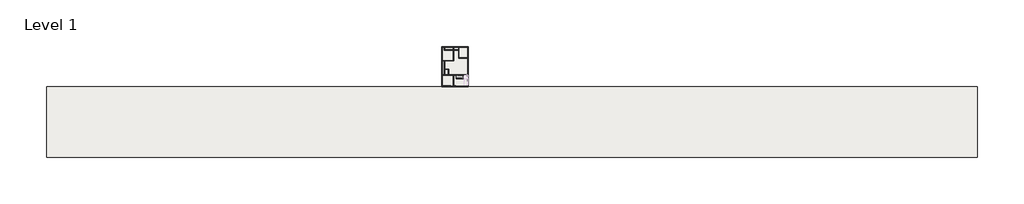
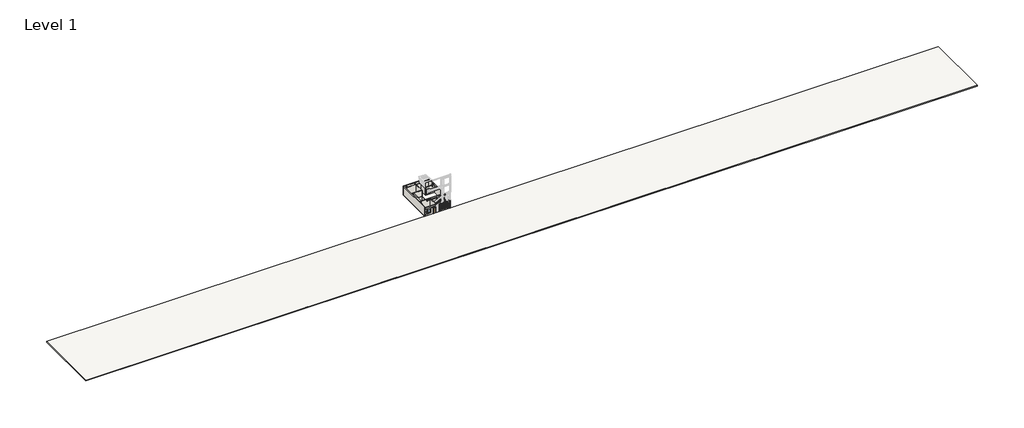
# One storey, part 1 of 2: 19 walls, 2 slabs, 1 door, 1 railing, 1 window.
"""IFC4 building model written with IfcOpenShell, lengths in millimetres."""

from ifc_helpers import new_model, si_unit, frame, origin, origin_with_axes, place, context, project, spatial, polyline, outline, extrude, faceted_brep, transform, mapped, element, save
from components import door_5e1232af, fixed_4x3_c1f32544

model = new_model("IFC4")

# Units and contexts
model_context = context("Model", 3, world=origin())
ifc_project = project(units=[si_unit("LENGTHUNIT", "METRE", prefix="MILLI")], contexts=[model_context])

# Site, building, storey
site = spatial("IfcSite", under=ifc_project)
building = spatial("IfcBuilding", under=site)
storey = spatial("IfcBuildingStorey", under=building, Name="Level 1", Elevation=0.0)

# Door
placement = place(None, origin())
door_shape = door_5e1232af(model_context)
element("IfcDoor", 1, ObjectType="Single-Flush : 30\" x 84\"", at=placement, inside=storey, context=model_context, shape_type="MappedRepresentation", body=[
    mapped(door_shape, transform((-2008.66646, -4503.4834702, 0.0), x_axis=(1.0, 0.0, 0.0), y_axis=(0.0, 1.0, 0.0), z_axis=(0.0, 0.0, 1.0))),
])

# Railing
element("IfcRailing", 2, ObjectType="Handrail - Rectangular", at=placement, inside=storey, context=model_context, shape_type="SolidModel", body=[
    faceted_brep([(-459.26646, -1798.3834702, 1066.8), (-459.26646, -1798.3834702, 1008.9343477), (-459.26646, -1849.1834702, 1008.9343477), (-459.26646, -1849.1834702, 1066.8), (2334.73354, -1798.3834702, 2590.8), (2347.687236, -1798.3834702, 2540.0), (2347.687236, -1849.1834702, 2540.0), (2334.73354, -1849.1834702, 2590.8), (2436.33354, -1798.3834702, 2590.8), (2436.33354, -1849.1834702, 2590.8), (2436.33354, -1849.1834702, 2540.0), (2436.33354, -1798.3834702, 2540.0)], [[[0, 1, 2, 3]], [[1, 0, 4, 5]], [[2, 1, 5, 6]], [[3, 2, 6, 7]], [[0, 3, 7, 4]], [[8, 9, 10, 11]], [[5, 4, 8, 11]], [[6, 5, 11, 10]], [[7, 6, 10, 9]], [[4, 7, 9, 8]]]),
    faceted_brep([(2436.33354, -1849.1834702, 2641.6), (2436.33354, -1849.1834702, 2528.0077467), (2385.53354, -1849.1834702, 2528.0077467), (2385.53354, -1849.1834702, 2641.6), (2436.33354, -1899.9834702, 2743.2), (2436.33354, -1938.2955084, 2706.231823), (2385.53354, -1938.2955084, 2706.231823), (2385.53354, -1899.9834702, 2743.2), (2436.33354, -4135.1834702, 3962.4), (2385.53354, -4135.1834702, 3962.4), (2385.53354, -4135.1834702, 3904.5343477), (2436.33354, -4135.1834702, 3904.5343477)], [[[0, 1, 2, 3]], [[1, 0, 4, 5]], [[2, 1, 5, 6]], [[3, 2, 6, 7]], [[0, 3, 7, 4]], [[8, 9, 10, 11]], [[5, 4, 8, 11]], [[6, 5, 11, 10]], [[7, 6, 10, 9]], [[4, 7, 9, 8]]]),
    extrude(outline(polyline([(-4043.1084702, 3854.3116204), (-4024.0584702, 3843.9207113), (-4024.0584702, 2895.6), (-4043.1084702, 2895.6), (-4043.1084702, 3854.3116204)])), frame((2401.40854, 0.0, 0.0), z_axis=(1.0, 0.0, 0.0), x_axis=(0.0, 1.0, 0.0)), (0.0, 0.0, 1.0), 19.05),
    extrude(outline(polyline([(-3941.5084702, 3798.8934386), (-3922.4584702, 3788.5025295), (-3922.4584702, 2895.6), (-3941.5084702, 2895.6), (-3941.5084702, 3798.8934386)])), frame((2401.40854, 0.0, 0.0), z_axis=(1.0, 0.0, 0.0), x_axis=(0.0, 1.0, 0.0)), (0.0, 0.0, 1.0), 19.05),
    extrude(outline(polyline([(-3839.9084702, 3743.4752568), (-3820.8584702, 3733.0843477), (-3820.8584702, 2743.2), (-3839.9084702, 2743.2), (-3839.9084702, 3743.4752568)])), frame((2401.40854, 0.0, 0.0), z_axis=(1.0, 0.0, 0.0), x_axis=(0.0, 1.0, 0.0)), (0.0, 0.0, 1.0), 19.05),
    extrude(outline(polyline([(-3738.3084702, 3688.0570749), (-3719.2584702, 3677.6661659), (-3719.2584702, 2743.2), (-3738.3084702, 2743.2), (-3738.3084702, 3688.0570749)])), frame((2401.40854, 0.0, 0.0), z_axis=(1.0, 0.0, 0.0), x_axis=(0.0, 1.0, 0.0)), (0.0, 0.0, 1.0), 19.05),
    extrude(outline(polyline([(-3636.7084702, 3632.6388931), (-3617.6584702, 3622.247984), (-3617.6584702, 2743.2), (-3636.7084702, 2743.2), (-3636.7084702, 3632.6388931)])), frame((2401.40854, 0.0, 0.0), z_axis=(1.0, 0.0, 0.0), x_axis=(0.0, 1.0, 0.0)), (0.0, 0.0, 1.0), 19.05),
    extrude(outline(polyline([(-3535.1084702, 3577.2207113), (-3516.0584702, 3566.8298022), (-3516.0584702, 2590.8), (-3535.1084702, 2590.8), (-3535.1084702, 3577.2207113)])), frame((2401.40854, 0.0, 0.0), z_axis=(1.0, 0.0, 0.0), x_axis=(0.0, 1.0, 0.0)), (0.0, 0.0, 1.0), 19.05),
    extrude(outline(polyline([(-3433.5084702, 3521.8025295), (-3414.4584702, 3511.4116204), (-3414.4584702, 2590.8), (-3433.5084702, 2590.8), (-3433.5084702, 3521.8025295)])), frame((2401.40854, 0.0, 0.0), z_axis=(1.0, 0.0, 0.0), x_axis=(0.0, 1.0, 0.0)), (0.0, 0.0, 1.0), 19.05),
    extrude(outline(polyline([(-3331.9084702, 3466.3843477), (-3312.8584702, 3455.9934386), (-3312.8584702, 2590.8), (-3331.9084702, 2590.8), (-3331.9084702, 3466.3843477)])), frame((2401.40854, 0.0, 0.0), z_axis=(1.0, 0.0, 0.0), x_axis=(0.0, 1.0, 0.0)), (0.0, 0.0, 1.0), 19.05),
    extrude(outline(polyline([(-3230.3084702, 3410.9661659), (-3211.2584702, 3400.5752568), (-3211.2584702, 2438.4), (-3230.3084702, 2438.4), (-3230.3084702, 3410.9661659)])), frame((2401.40854, 0.0, 0.0), z_axis=(1.0, 0.0, 0.0), x_axis=(0.0, 1.0, 0.0)), (0.0, 0.0, 1.0), 19.05),
    extrude(outline(polyline([(-3128.7084702, 3355.547984), (-3109.6584702, 3345.1570749), (-3109.6584702, 2438.4), (-3128.7084702, 2438.4), (-3128.7084702, 3355.547984)])), frame((2401.40854, 0.0, 0.0), z_axis=(1.0, 0.0, 0.0), x_axis=(0.0, 1.0, 0.0)), (0.0, 0.0, 1.0), 19.05),
    extrude(outline(polyline([(-3027.1084702, 3300.1298022), (-3008.0584702, 3289.7388931), (-3008.0584702, 2438.4), (-3027.1084702, 2438.4), (-3027.1084702, 3300.1298022)])), frame((2401.40854, 0.0, 0.0), z_axis=(1.0, 0.0, 0.0), x_axis=(0.0, 1.0, 0.0)), (0.0, 0.0, 1.0), 19.05),
    extrude(outline(polyline([(-2925.5084702, 3244.7116204), (-2906.4584702, 3234.3207113), (-2906.4584702, 2286.0), (-2925.5084702, 2286.0), (-2925.5084702, 3244.7116204)])), frame((2401.40854, 0.0, 0.0), z_axis=(1.0, 0.0, 0.0), x_axis=(0.0, 1.0, 0.0)), (0.0, 0.0, 1.0), 19.05),
    extrude(outline(polyline([(-2823.9084702, 3189.2934386), (-2804.8584702, 3178.9025295), (-2804.8584702, 2286.0), (-2823.9084702, 2286.0), (-2823.9084702, 3189.2934386)])), frame((2401.40854, 0.0, 0.0), z_axis=(1.0, 0.0, 0.0), x_axis=(0.0, 1.0, 0.0)), (0.0, 0.0, 1.0), 19.05),
    extrude(outline(polyline([(-2722.3084702, 3133.8752568), (-2703.2584702, 3123.4843477), (-2703.2584702, 2133.6), (-2722.3084702, 2133.6), (-2722.3084702, 3133.8752568)])), frame((2401.40854, 0.0, 0.0), z_axis=(1.0, 0.0, 0.0), x_axis=(0.0, 1.0, 0.0)), (0.0, 0.0, 1.0), 19.05),
    extrude(outline(polyline([(-2620.7084702, 3078.4570749), (-2601.6584702, 3068.0661659), (-2601.6584702, 2133.6), (-2620.7084702, 2133.6), (-2620.7084702, 3078.4570749)])), frame((2401.40854, 0.0, 0.0), z_axis=(1.0, 0.0, 0.0), x_axis=(0.0, 1.0, 0.0)), (0.0, 0.0, 1.0), 19.05),
    extrude(outline(polyline([(-2519.1084702, 3023.0388931), (-2500.0584702, 3012.647984), (-2500.0584702, 2133.6), (-2519.1084702, 2133.6), (-2519.1084702, 3023.0388931)])), frame((2401.40854, 0.0, 0.0), z_axis=(1.0, 0.0, 0.0), x_axis=(0.0, 1.0, 0.0)), (0.0, 0.0, 1.0), 19.05),
    extrude(outline(polyline([(-2417.5084702, 2967.6207113), (-2398.4584702, 2957.2298022), (-2398.4584702, 1981.2), (-2417.5084702, 1981.2), (-2417.5084702, 2967.6207113)])), frame((2401.40854, 0.0, 0.0), z_axis=(1.0, 0.0, 0.0), x_axis=(0.0, 1.0, 0.0)), (0.0, 0.0, 1.0), 19.05),
    extrude(outline(polyline([(-2315.9084702, 2912.2025295), (-2296.8584702, 2901.8116204), (-2296.8584702, 1981.2), (-2315.9084702, 1981.2), (-2315.9084702, 2912.2025295)])), frame((2401.40854, 0.0, 0.0), z_axis=(1.0, 0.0, 0.0), x_axis=(0.0, 1.0, 0.0)), (0.0, 0.0, 1.0), 19.05),
    extrude(outline(polyline([(-2214.3084702, 2856.7843477), (-2195.2584702, 2846.3934386), (-2195.2584702, 1981.2), (-2214.3084702, 1981.2), (-2214.3084702, 2856.7843477)])), frame((2401.40854, 0.0, 0.0), z_axis=(1.0, 0.0, 0.0), x_axis=(0.0, 1.0, 0.0)), (0.0, 0.0, 1.0), 19.05),
    extrude(outline(polyline([(-2112.7084702, 2801.3661659), (-2093.6584702, 2790.9752568), (-2093.6584702, 1828.8), (-2112.7084702, 1828.8), (-2112.7084702, 2801.3661659)])), frame((2401.40854, 0.0, 0.0), z_axis=(1.0, 0.0, 0.0), x_axis=(0.0, 1.0, 0.0)), (0.0, 0.0, 1.0), 19.05),
    extrude(outline(polyline([(-2011.1084702, 2745.947984), (-1992.0584702, 2735.5570749), (-1992.0584702, 1828.8), (-2011.1084702, 1828.8), (-2011.1084702, 2745.947984)])), frame((2401.40854, 0.0, 0.0), z_axis=(1.0, 0.0, 0.0), x_axis=(0.0, 1.0, 0.0)), (0.0, 0.0, 1.0), 19.05),
    extrude(outline(polyline([(2510.4207113, 2293.45854), (2500.0298022, 2274.40854), (1524.0, 2274.40854), (1524.0, 2293.45854), (2510.4207113, 2293.45854)])), frame((0.0, -1833.3084702, 0.0), z_axis=(0.0, 1.0, 0.0), x_axis=(0.0, 0.0, 1.0)), (0.0, 0.0, 1.0), 19.05),
    extrude(outline(polyline([(2455.0025295, 2191.85854), (2444.6116204, 2172.80854), (1524.0, 2172.80854), (1524.0, 2191.85854), (2455.0025295, 2191.85854)])), frame((0.0, -1833.3084702, 0.0), z_axis=(0.0, 1.0, 0.0), x_axis=(0.0, 0.0, 1.0)), (0.0, 0.0, 1.0), 19.05),
    extrude(outline(polyline([(2399.5843477, 2090.25854), (2389.1934386, 2071.20854), (1524.0, 2071.20854), (1524.0, 2090.25854), (2399.5843477, 2090.25854)])), frame((0.0, -1833.3084702, 0.0), z_axis=(0.0, 1.0, 0.0), x_axis=(0.0, 0.0, 1.0)), (0.0, 0.0, 1.0), 19.05),
    extrude(outline(polyline([(2344.1661659, 1988.65854), (2333.7752568, 1969.60854), (1371.6, 1969.60854), (1371.6, 1988.65854), (2344.1661659, 1988.65854)])), frame((0.0, -1833.3084702, 0.0), z_axis=(0.0, 1.0, 0.0), x_axis=(0.0, 0.0, 1.0)), (0.0, 0.0, 1.0), 19.05),
    extrude(outline(polyline([(2288.747984, 1887.05854), (2278.3570749, 1868.00854), (1371.6, 1868.00854), (1371.6, 1887.05854), (2288.747984, 1887.05854)])), frame((0.0, -1833.3084702, 0.0), z_axis=(0.0, 1.0, 0.0), x_axis=(0.0, 0.0, 1.0)), (0.0, 0.0, 1.0), 19.05),
    extrude(outline(polyline([(2233.3298022, 1785.45854), (2222.9388931, 1766.40854), (1371.6, 1766.40854), (1371.6, 1785.45854), (2233.3298022, 1785.45854)])), frame((0.0, -1833.3084702, 0.0), z_axis=(0.0, 1.0, 0.0), x_axis=(0.0, 0.0, 1.0)), (0.0, 0.0, 1.0), 19.05),
    extrude(outline(polyline([(2177.9116204, 1683.85854), (2167.5207113, 1664.80854), (1219.2, 1664.80854), (1219.2, 1683.85854), (2177.9116204, 1683.85854)])), frame((0.0, -1833.3084702, 0.0), z_axis=(0.0, 1.0, 0.0), x_axis=(0.0, 0.0, 1.0)), (0.0, 0.0, 1.0), 19.05),
    extrude(outline(polyline([(2122.4934386, 1582.25854), (2112.1025295, 1563.20854), (1219.2, 1563.20854), (1219.2, 1582.25854), (2122.4934386, 1582.25854)])), frame((0.0, -1833.3084702, 0.0), z_axis=(0.0, 1.0, 0.0), x_axis=(0.0, 0.0, 1.0)), (0.0, 0.0, 1.0), 19.05),
    extrude(outline(polyline([(2067.0752568, 1480.65854), (2056.6843477, 1461.60854), (1066.8, 1461.60854), (1066.8, 1480.65854), (2067.0752568, 1480.65854)])), frame((0.0, -1833.3084702, 0.0), z_axis=(0.0, 1.0, 0.0), x_axis=(0.0, 0.0, 1.0)), (0.0, 0.0, 1.0), 19.05),
    extrude(outline(polyline([(2011.6570749, 1379.05854), (2001.2661659, 1360.00854), (1066.8, 1360.00854), (1066.8, 1379.05854), (2011.6570749, 1379.05854)])), frame((0.0, -1833.3084702, 0.0), z_axis=(0.0, 1.0, 0.0), x_axis=(0.0, 0.0, 1.0)), (0.0, 0.0, 1.0), 19.05),
    extrude(outline(polyline([(1956.2388931, 1277.45854), (1945.847984, 1258.40854), (1066.8, 1258.40854), (1066.8, 1277.45854), (1956.2388931, 1277.45854)])), frame((0.0, -1833.3084702, 0.0), z_axis=(0.0, 1.0, 0.0), x_axis=(0.0, 0.0, 1.0)), (0.0, 0.0, 1.0), 19.05),
    extrude(outline(polyline([(1900.8207113, 1175.85854), (1890.4298022, 1156.80854), (914.4, 1156.80854), (914.4, 1175.85854), (1900.8207113, 1175.85854)])), frame((0.0, -1833.3084702, 0.0), z_axis=(0.0, 1.0, 0.0), x_axis=(0.0, 0.0, 1.0)), (0.0, 0.0, 1.0), 19.05),
    extrude(outline(polyline([(1845.4025295, 1074.25854), (1835.0116204, 1055.20854), (914.4, 1055.20854), (914.4, 1074.25854), (1845.4025295, 1074.25854)])), frame((0.0, -1833.3084702, 0.0), z_axis=(0.0, 1.0, 0.0), x_axis=(0.0, 0.0, 1.0)), (0.0, 0.0, 1.0), 19.05),
    extrude(outline(polyline([(1789.9843477, 972.65854), (1779.5934386, 953.60854), (914.4, 953.60854), (914.4, 972.65854), (1789.9843477, 972.65854)])), frame((0.0, -1833.3084702, 0.0), z_axis=(0.0, 1.0, 0.0), x_axis=(0.0, 0.0, 1.0)), (0.0, 0.0, 1.0), 19.05),
    extrude(outline(polyline([(1734.5661659, 871.05854), (1724.1752568, 852.00854), (762.0, 852.00854), (762.0, 871.05854), (1734.5661659, 871.05854)])), frame((0.0, -1833.3084702, 0.0), z_axis=(0.0, 1.0, 0.0), x_axis=(0.0, 0.0, 1.0)), (0.0, 0.0, 1.0), 19.05),
    extrude(outline(polyline([(1679.147984, 769.45854), (1668.7570749, 750.40854), (762.0, 750.40854), (762.0, 769.45854), (1679.147984, 769.45854)])), frame((0.0, -1833.3084702, 0.0), z_axis=(0.0, 1.0, 0.0), x_axis=(0.0, 0.0, 1.0)), (0.0, 0.0, 1.0), 19.05),
    extrude(outline(polyline([(1623.7298022, 667.85854), (1613.3388931, 648.80854), (762.0, 648.80854), (762.0, 667.85854), (1623.7298022, 667.85854)])), frame((0.0, -1833.3084702, 0.0), z_axis=(0.0, 1.0, 0.0), x_axis=(0.0, 0.0, 1.0)), (0.0, 0.0, 1.0), 19.05),
    extrude(outline(polyline([(1568.3116204, 566.25854), (1557.9207113, 547.20854), (609.6, 547.20854), (609.6, 566.25854), (1568.3116204, 566.25854)])), frame((0.0, -1833.3084702, 0.0), z_axis=(0.0, 1.0, 0.0), x_axis=(0.0, 0.0, 1.0)), (0.0, 0.0, 1.0), 19.05),
    extrude(outline(polyline([(1512.8934386, 464.65854), (1502.5025295, 445.60854), (609.6, 445.60854), (609.6, 464.65854), (1512.8934386, 464.65854)])), frame((0.0, -1833.3084702, 0.0), z_axis=(0.0, 1.0, 0.0), x_axis=(0.0, 0.0, 1.0)), (0.0, 0.0, 1.0), 19.05),
    extrude(outline(polyline([(1457.4752568, 363.05854), (1447.0843477, 344.00854), (457.2, 344.00854), (457.2, 363.05854), (1457.4752568, 363.05854)])), frame((0.0, -1833.3084702, 0.0), z_axis=(0.0, 1.0, 0.0), x_axis=(0.0, 0.0, 1.0)), (0.0, 0.0, 1.0), 19.05),
    extrude(outline(polyline([(1402.0570749, 261.45854), (1391.6661659, 242.40854), (457.2, 242.40854), (457.2, 261.45854), (1402.0570749, 261.45854)])), frame((0.0, -1833.3084702, 0.0), z_axis=(0.0, 1.0, 0.0), x_axis=(0.0, 0.0, 1.0)), (0.0, 0.0, 1.0), 19.05),
    extrude(outline(polyline([(1346.6388931, 159.85854), (1336.247984, 140.80854), (457.2, 140.80854), (457.2, 159.85854), (1346.6388931, 159.85854)])), frame((0.0, -1833.3084702, 0.0), z_axis=(0.0, 1.0, 0.0), x_axis=(0.0, 0.0, 1.0)), (0.0, 0.0, 1.0), 19.05),
    extrude(outline(polyline([(1291.2207113, 58.25854), (1280.8298022, 39.20854), (304.8, 39.20854), (304.8, 58.25854), (1291.2207113, 58.25854)])), frame((0.0, -1833.3084702, 0.0), z_axis=(0.0, 1.0, 0.0), x_axis=(0.0, 0.0, 1.0)), (0.0, 0.0, 1.0), 19.05),
    extrude(outline(polyline([(1235.8025295, -43.34146), (1225.4116204, -62.39146), (304.8, -62.39146), (304.8, -43.34146), (1235.8025295, -43.34146)])), frame((0.0, -1833.3084702, 0.0), z_axis=(0.0, 1.0, 0.0), x_axis=(0.0, 0.0, 1.0)), (0.0, 0.0, 1.0), 19.05),
    extrude(outline(polyline([(1180.3843477, -144.94146), (1169.9934386, -163.99146), (304.8, -163.99146), (304.8, -144.94146), (1180.3843477, -144.94146)])), frame((0.0, -1833.3084702, 0.0), z_axis=(0.0, 1.0, 0.0), x_axis=(0.0, 0.0, 1.0)), (0.0, 0.0, 1.0), 19.05),
    extrude(outline(polyline([(1124.9661659, -246.54146), (1114.5752568, -265.59146), (152.4, -265.59146), (152.4, -246.54146), (1124.9661659, -246.54146)])), frame((0.0, -1833.3084702, 0.0), z_axis=(0.0, 1.0, 0.0), x_axis=(0.0, 0.0, 1.0)), (0.0, 0.0, 1.0), 19.05),
    extrude(outline(polyline([(1069.547984, -348.14146), (1059.1570749, -367.19146), (152.4, -367.19146), (152.4, -348.14146), (1069.547984, -348.14146)])), frame((0.0, -1833.3084702, 0.0), z_axis=(0.0, 1.0, 0.0), x_axis=(0.0, 0.0, 1.0)), (0.0, 0.0, 1.0), 19.05),
    extrude(outline(polyline([(-1909.5084702, 2648.6577467), (-1890.4584702, 2610.5577467), (-1890.4584702, 1676.4), (-1909.5084702, 1676.4), (-1909.5084702, 2648.6577467)])), frame((2401.40854, 0.0, 0.0), z_axis=(1.0, 0.0, 0.0), x_axis=(0.0, 1.0, 0.0)), (0.0, 0.0, 1.0), 19.05),
    extrude(outline(polyline([(2401.40854, -1833.3084702), (2401.40854, -1814.2584702), (2420.45854, -1814.2584702), (2420.45854, -1833.3084702), (2401.40854, -1833.3084702)])), frame((0.0, 0.0, 1676.4), z_axis=(0.0, 0.0, 1.0), x_axis=(1.0, 0.0, 0.0)), (0.0, 0.0, 1.0), 863.6),
    extrude(outline(polyline([(2538.1298022, 2344.25854), (2527.7388931, 2325.20854), (1676.4, 2325.20854), (1676.4, 2344.25854), (2538.1298022, 2344.25854)])), frame((0.0, -1833.3084702, 0.0), z_axis=(0.0, 1.0, 0.0), x_axis=(0.0, 0.0, 1.0)), (0.0, 0.0, 1.0), 19.05),
    extrude(outline(polyline([(-4135.1834702, 3904.5343477), (-4116.1334702, 3894.1434386), (-4116.1334702, 2895.6), (-4135.1834702, 2895.6), (-4135.1834702, 3904.5343477)])), frame((2401.40854, 0.0, 0.0), z_axis=(1.0, 0.0, 0.0), x_axis=(0.0, 1.0, 0.0)), (0.0, 0.0, 1.0), 19.05),
    extrude(outline(polyline([(1019.3252568, -440.21646), (1008.9343477, -459.26646), (152.4, -459.26646), (152.4, -440.21646), (1019.3252568, -440.21646)])), frame((0.0, -1833.3084702, 0.0), z_axis=(0.0, 1.0, 0.0), x_axis=(0.0, 0.0, 1.0)), (0.0, 0.0, 1.0), 19.05),
])

# Slabs
element("IfcSlab", 3, ObjectType="Generic - 12\"", at=placement, inside=storey, context=model_context, shape_type="SweptSolid", body=[
    extrude(outline(polyline([(3757.13354, 9098.2165298), (3757.13354, -4617.7834702), (-5386.86646, -4617.7834702), (-5386.86646, 9098.2165298), (3757.13354, 9098.2165298)]), holes=[polyline([(-4548.66646, 4170.6165298), (-5158.26646, 4170.6165298), (-5158.26646, -604.5834702), (-4548.66646, -604.5834702), (-4548.66646, 4170.6165298)]), polyline([(353.53354, 8869.6165298), (-1373.66646, 8869.6165298), (-1373.66646, 7955.2165298), (353.53354, 7955.2165298), (353.53354, 8869.6165298)])]), frame((0.0, 0.0, -304.8), z_axis=(0.0, 0.0, 1.0), x_axis=(1.0, 0.0, 0.0)), (0.0, 0.0, 1.0), 304.8),
])
element("IfcSlab", 4, ObjectType="Generic - 12\"", at=placement, inside=storey, context=model_context, shape_type="SweptSolid", body=[
    extrude(outline(polyline([(178408.3047378, -4668.5834702), (178408.3047378, -28877.350551), (-141022.0952622, -28877.350551), (-141022.0952622, -4668.5834702), (178408.3047378, -4668.5834702)])), frame((0.0, 0.0, -304.8), z_axis=(0.0, 0.0, 1.0), x_axis=(1.0, 0.0, 0.0)), (0.0, 0.0, 1.0), 304.8),
])

# Walls
element("IfcWall", 5, ObjectType="Generic - 5\"", at=placement, inside=storey, context=model_context, shape_type="Brep", body=[
    faceted_brep([(-1373.66646, -4389.1834702, 0.0), (-1373.66646, -731.5834702, 0.0), (-1373.66646, -604.5834702, 0.0), (-1373.66646, -604.5834702, 3048.0), (-1373.66646, -731.5834702, 3048.0), (-1373.66646, -4389.1834702, 3048.0), (-1500.66646, -4389.1834702, 0.0), (-1500.66646, -4389.1834702, 3048.0), (-1500.66646, -731.5834702, 3048.0), (-1500.66646, -604.5834702, 3048.0), (-1500.66646, -604.5834702, 0.0), (-1500.66646, -731.5834702, 0.0)], [[[0, 1, 2, 3, 4, 5]], [[6, 7, 8, 9, 10, 11]], [[2, 1, 0, 6, 11, 10]], [[5, 4, 3, 9, 8, 7]], [[0, 5, 7, 6]], [[3, 2, 10, 9]]]),
])
element("IfcWall", 6, ObjectType="Generic - 5\"", at=placement, inside=storey, context=model_context, shape_type="Brep", body=[
    faceted_brep([(-1500.66646, -604.5834702, 0.0), (-3075.46646, -604.5834702, 0.0), (-3202.46646, -604.5834702, 0.0), (-4421.66646, -604.5834702, 0.0), (-4548.66646, -604.5834702, 0.0), (-5158.26646, -604.5834702, 0.0), (-5158.26646, -604.5834702, 3048.0), (-4548.66646, -604.5834702, 3048.0), (-4421.66646, -604.5834702, 3048.0), (-3202.46646, -604.5834702, 3048.0), (-3075.46646, -604.5834702, 3048.0), (-1500.66646, -604.5834702, 3048.0), (-1500.66646, -731.5834702, 0.0), (-1500.66646, -731.5834702, 3048.0), (-5158.26646, -731.5834702, 3048.0), (-5158.26646, -731.5834702, 0.0)], [[[0, 1, 2, 3, 4, 5, 6, 7, 8, 9, 10, 11]], [[12, 13, 14, 15]], [[5, 4, 3, 2, 1, 0, 12, 15]], [[11, 10, 9, 8, 7, 6, 14, 13]], [[0, 11, 13, 12]], [[6, 5, 15, 14]]]),
])
element("IfcWall", 7, ObjectType="Generic - 5\"", at=placement, inside=storey, context=model_context, shape_type="SweptSolid", body=[
    extrude(outline(polyline([(3528.53354, -731.5834702), (-1373.66646, -731.5834702), (-1373.66646, -604.5834702), (3528.53354, -604.5834702), (3528.53354, -731.5834702)])), origin_with_axes(), (0.0, 0.0, 1.0), 3048.0),
])
element("IfcWall", 8, ObjectType="Generic - 5\"", at=placement, inside=storey, context=model_context, shape_type="Brep", body=[
    faceted_brep([(-1500.66646, 8869.6165298, 0.0), (-1500.66646, 7955.2165298, 0.0), (-1500.66646, 7828.2165298, 0.0), (-1500.66646, 4297.6165298, 0.0), (-1500.66646, 4170.6165298, 0.0), (-1500.66646, 4170.6165298, 3048.0), (-1500.66646, 4297.6165298, 3048.0), (-1500.66646, 7828.2165298, 3048.0), (-1500.66646, 7955.2165298, 3048.0), (-1500.66646, 8869.6165298, 3048.0), (-1373.66646, 8869.6165298, 0.0), (-1373.66646, 8869.6165298, 3048.0), (-1373.66646, 7955.2165298, 3048.0), (-1373.66646, 7828.2165298, 3048.0), (-1373.66646, 4170.6165298, 3048.0), (-1373.66646, 4170.6165298, 0.0), (-1373.66646, 7828.2165298, 0.0), (-1373.66646, 7955.2165298, 0.0)], [[[0, 1, 2, 3, 4, 5, 6, 7, 8, 9]], [[10, 11, 12, 13, 14, 15, 16, 17]], [[4, 3, 2, 1, 0, 10, 17, 16, 15]], [[9, 8, 7, 6, 5, 14, 13, 12, 11]], [[0, 9, 11, 10]], [[5, 4, 15, 14]]]),
])
element("IfcWall", 9, ObjectType="Generic - 5\"", at=placement, inside=storey, context=model_context, shape_type="Brep", body=[
    faceted_brep([(-1500.66646, 4297.6165298, 0.0), (-5158.26646, 4297.6165298, 0.0), (-5158.26646, 4297.6165298, 3048.0), (-1500.66646, 4297.6165298, 3048.0), (-1500.66646, 4170.6165298, 0.0), (-1500.66646, 4170.6165298, 3048.0), (-4421.66646, 4170.6165298, 3048.0), (-4548.66646, 4170.6165298, 3048.0), (-5158.26646, 4170.6165298, 3048.0), (-5158.26646, 4170.6165298, 0.0), (-4548.66646, 4170.6165298, 0.0), (-4421.66646, 4170.6165298, 0.0)], [[[0, 1, 2, 3]], [[4, 5, 6, 7, 8, 9, 10, 11]], [[1, 0, 4, 11, 10, 9]], [[3, 2, 8, 7, 6, 5]], [[0, 3, 5, 4]], [[2, 1, 9, 8]]]),
])
element("IfcWall", 10, ObjectType="Generic - 5\"", at=placement, inside=storey, context=model_context, shape_type="Brep", body=[
    faceted_brep([(353.53354, 8869.6165298, 0.0), (353.53354, 7955.2165298, 0.0), (353.53354, 7828.2165298, 0.0), (353.53354, 7828.2165298, 3048.0), (353.53354, 7955.2165298, 3048.0), (353.53354, 8869.6165298, 3048.0), (480.53354, 8869.6165298, 0.0), (480.53354, 8869.6165298, 3048.0), (480.53354, 7828.2165298, 3048.0), (480.53354, 7828.2165298, 0.0)], [[[0, 1, 2, 3, 4, 5]], [[6, 7, 8, 9]], [[2, 1, 0, 6, 9]], [[5, 4, 3, 8, 7]], [[0, 5, 7, 6]], [[3, 2, 9, 8]]]),
])
element("IfcWall", 11, ObjectType="Generic - 5\"", at=placement, inside=storey, context=model_context, shape_type="SweptSolid", body=[
    extrude(outline(polyline([(-1373.66646, 7955.2165298), (353.53354, 7955.2165298), (353.53354, 7828.2165298), (-1373.66646, 7828.2165298), (-1373.66646, 7955.2165298)])), origin_with_axes(), (0.0, 0.0, 1.0), 3048.0),
])
element("IfcWall", 12, ObjectType="Generic - 5\"", at=placement, inside=storey, context=model_context, shape_type="Brep", body=[
    faceted_brep([(3528.53354, 5212.0165298, 0.0), (480.53354, 5212.0165298, 0.0), (353.53354, 5212.0165298, 0.0), (353.53354, 5212.0165298, 3048.0), (480.53354, 5212.0165298, 3048.0), (3528.53354, 5212.0165298, 3048.0), (3528.53354, 5085.0165298, 0.0), (3528.53354, 5085.0165298, 3048.0), (353.53354, 5085.0165298, 3048.0), (353.53354, 5085.0165298, 0.0)], [[[0, 1, 2, 3, 4, 5]], [[6, 7, 8, 9]], [[2, 1, 0, 6, 9]], [[5, 4, 3, 8, 7]], [[0, 5, 7, 6]], [[3, 2, 9, 8]]]),
])
element("IfcWall", 13, ObjectType="Generic - 5\"", at=placement, inside=storey, context=model_context, shape_type="SweptSolid", body=[
    extrude(outline(polyline([(480.53354, 7828.2165298), (480.53354, 5212.0165298), (353.53354, 5212.0165298), (353.53354, 7828.2165298), (480.53354, 7828.2165298)])), origin_with_axes(), (0.0, 0.0, 1.0), 3048.0),
])
element("IfcWall", 14, ObjectType="Generic - 5\"", at=placement, inside=storey, context=model_context, shape_type="Brep", body=[
    faceted_brep([(-4421.66646, -604.5834702, 0.0), (-4421.66646, 1224.2165298, 0.0), (-4421.66646, 1351.2165298, 0.0), (-4421.66646, 4170.6165298, 0.0), (-4421.66646, 4170.6165298, 3048.0), (-4421.66646, 1351.2165298, 3048.0), (-4421.66646, 1224.2165298, 3048.0), (-4421.66646, -604.5834702, 3048.0), (-4548.66646, -604.5834702, 0.0), (-4548.66646, -604.5834702, 3048.0), (-4548.66646, 4170.6165298, 3048.0), (-4548.66646, 4170.6165298, 0.0)], [[[0, 1, 2, 3, 4, 5, 6, 7]], [[8, 9, 10, 11]], [[3, 2, 1, 0, 8, 11]], [[7, 6, 5, 4, 10, 9]], [[0, 7, 9, 8]], [[4, 3, 11, 10]]]),
])
element("IfcWall", 15, ObjectType="Generic - 5\"", at=placement, inside=storey, context=model_context, shape_type="Brep", body=[
    faceted_brep([(-3075.46646, -604.5834702, 0.0), (-3075.46646, 1351.2165298, 0.0), (-3075.46646, 1351.2165298, 3048.0), (-3075.46646, -604.5834702, 3048.0), (-3202.46646, -604.5834702, 0.0), (-3202.46646, -604.5834702, 3048.0), (-3202.46646, 1224.2165298, 3048.0), (-3202.46646, 1351.2165298, 3048.0), (-3202.46646, 1351.2165298, 0.0), (-3202.46646, 1224.2165298, 0.0)], [[[0, 1, 2, 3]], [[4, 5, 6, 7, 8, 9]], [[1, 0, 4, 9, 8]], [[3, 2, 7, 6, 5]], [[0, 3, 5, 4]], [[2, 1, 8, 7]]]),
])
element("IfcWall", 16, ObjectType="Generic - 5\"", at=placement, inside=storey, context=model_context, shape_type="SweptSolid", body=[
    extrude(outline(polyline([(-4421.66646, 1351.2165298), (-3202.46646, 1351.2165298), (-3202.46646, 1224.2165298), (-4421.66646, 1224.2165298), (-4421.66646, 1351.2165298)])), origin_with_axes(), (0.0, 0.0, 1.0), 3048.0),
])
element("IfcWall", 17, ObjectType="Generic - 5\"", at=placement, inside=storey, context=model_context, shape_type="Brep", body=[
    faceted_brep([(-1500.66646, 7955.2165298, 0.0), (-4421.66646, 7955.2165298, 0.0), (-4548.66646, 7955.2165298, 0.0), (-4548.66646, 7955.2165298, 3048.0), (-4421.66646, 7955.2165298, 3048.0), (-1500.66646, 7955.2165298, 3048.0), (-1500.66646, 7828.2165298, 0.0), (-1500.66646, 7828.2165298, 3048.0), (-4548.66646, 7828.2165298, 3048.0), (-4548.66646, 7828.2165298, 0.0)], [[[0, 1, 2, 3, 4, 5]], [[6, 7, 8, 9]], [[2, 1, 0, 6, 9]], [[5, 4, 3, 8, 7]], [[0, 5, 7, 6]], [[3, 2, 9, 8]]]),
])
element("IfcWall", 18, ObjectType="Generic - 5\"", at=placement, inside=storey, context=model_context, shape_type="SweptSolid", body=[
    extrude(outline(polyline([(-4421.66646, 8869.6165298), (-4421.66646, 7955.2165298), (-4548.66646, 7955.2165298), (-4548.66646, 8869.6165298), (-4421.66646, 8869.6165298)])), origin_with_axes(), (0.0, 0.0, 1.0), 3048.0),
])
element("IfcWall", 19, ObjectType="Generic - 5\"", at=placement, inside=storey, context=model_context, shape_type="SweptSolid", body=[
    extrude(outline(polyline([(2438.4, -618.6794792), (2438.4, 1482.2803125), (2438.4, 3527.8705208), (3048.0, 3527.8705208), (3048.0, 1468.8712754), (3048.0, -618.6794792), (2438.4, -618.6794792)]), holes=[polyline([(2905.3237927, 3221.4816896), (2854.5237927, 3221.4816896), (2854.5237927, -410.7183104), (2905.3237927, -410.7183104), (2905.3237927, 3221.4816896)]), polyline([(2752.9237927, 3221.4816896), (2702.1237927, 3221.4816896), (2702.1237927, -410.7183104), (2752.9237927, -410.7183104), (2752.9237927, 3221.4816896)]), polyline([(2625.9237927, 3221.4816896), (2575.1237927, 3221.4816896), (2575.1237927, -410.7183104), (2625.9237927, -410.7183104), (2625.9237927, 3221.4816896)])]), frame((0.0, -4617.7834702, 0.0), z_axis=(0.0, 1.0, 0.0), x_axis=(0.0, 0.0, 1.0)), (0.0, 0.0, 1.0), 127.0),
    extrude(outline(polyline([(0.0, 1429.1955208), (2387.6, 1429.1955208), (2387.6, -618.6794792), (0.0, -618.6794792), (0.0, 1429.1955208)]), holes=[polyline([(2088.2821154, 870.7973513), (2088.2821154, 1023.1973513), (411.8821154, 1023.1973513), (411.8821154, 870.7973513), (2088.2821154, 870.7973513)]), polyline([(2088.2821154, 480.53354), (2088.2821154, 632.93354), (411.8821154, 632.93354), (411.8821154, 480.53354), (2088.2821154, 480.53354)]), polyline([(2088.2821154, 99.53354), (2088.2821154, 251.93354), (411.8821154, 251.93354), (411.8821154, 99.53354), (2088.2821154, 99.53354)]), polyline([(2088.2821154, -281.46646), (2088.2821154, -129.06646), (411.8821154, -129.06646), (411.8821154, -281.46646), (2088.2821154, -281.46646)])]), frame((0.0, -4617.7834702, 0.0), z_axis=(0.0, 1.0, 0.0), x_axis=(0.0, 0.0, 1.0)), (0.0, 0.0, 1.0), 127.0),
    extrude(outline(polyline([(2387.6, 1479.9955208), (0.0, 1479.9955208), (0.0, 3527.8705208), (2387.6, 3527.8705208), (2387.6, 1479.9955208)]), holes=[polyline([(2088.2821154, 2038.3936902), (411.8821154, 2038.3936902), (411.8821154, 1885.9936902), (2088.2821154, 1885.9936902), (2088.2821154, 2038.3936902)]), polyline([(2088.2821154, 2428.6575015), (411.8821154, 2428.6575015), (411.8821154, 2276.2575015), (2088.2821154, 2276.2575015), (2088.2821154, 2428.6575015)]), polyline([(2088.2821154, 2809.6575015), (411.8821154, 2809.6575015), (411.8821154, 2657.2575015), (2088.2821154, 2657.2575015), (2088.2821154, 2809.6575015)]), polyline([(2088.2821154, 3190.6575015), (411.8821154, 3190.6575015), (411.8821154, 3038.2575015), (2088.2821154, 3038.2575015), (2088.2821154, 3190.6575015)])]), frame((0.0, -4617.7834702, 0.0), z_axis=(0.0, 1.0, 0.0), x_axis=(0.0, 0.0, 1.0)), (0.0, 0.0, 1.0), 127.0),
])
element("IfcWall", 20, ObjectType="Generic -9\"", at=placement, inside=storey, context=model_context, shape_type="Brep", body=[
    faceted_brep([(-5386.86646, 8869.6165298, 0.0), (-5158.26646, 8869.6165298, 0.0), (-4548.66646, 8869.6165298, 0.0), (-4421.66646, 8869.6165298, 0.0), (-1500.66646, 8869.6165298, 0.0), (-1373.66646, 8869.6165298, 0.0), (353.53354, 8869.6165298, 0.0), (480.53354, 8869.6165298, 0.0), (3528.53354, 8869.6165298, 0.0), (3757.13354, 8869.6165298, 0.0), (3757.13354, 8869.6165298, 3048.0), (3528.53354, 8869.6165298, 3048.0), (480.53354, 8869.6165298, 3048.0), (353.53354, 8869.6165298, 3048.0), (-1373.66646, 8869.6165298, 3048.0), (-1500.66646, 8869.6165298, 3048.0), (-4421.66646, 8869.6165298, 3048.0), (-4548.66646, 8869.6165298, 3048.0), (-5158.26646, 8869.6165298, 3048.0), (-5386.86646, 8869.6165298, 3048.0), (-5386.86646, 9098.2165298, 0.0), (-5386.86646, 9098.2165298, 3048.0), (3757.13354, 9098.2165298, 3048.0), (3757.13354, 9098.2165298, 0.0)], [[[0, 1, 2, 3, 4, 5, 6, 7, 8, 9, 10, 11, 12, 13, 14, 15, 16, 17, 18, 19]], [[20, 21, 22, 23]], [[9, 8, 7, 6, 5, 4, 3, 2, 1, 0, 20, 23]], [[19, 18, 17, 16, 15, 14, 13, 12, 11, 10, 22, 21]], [[10, 9, 23, 22]], [[0, 19, 21, 20]]]),
])
element("IfcWall", 21, ObjectType="Generic -9\"", at=placement, inside=storey, context=model_context, shape_type="Brep", body=[
    faceted_brep([(3528.53354, 8869.6165298, 0.0), (3528.53354, 5212.0165298, 0.0), (3528.53354, 5085.0165298, 0.0), (3528.53354, -604.5834702, 0.0), (3528.53354, -731.5834702, 0.0), (3528.53354, -4617.7834702, 0.0), (3528.53354, -4617.7834702, 3048.0), (3528.53354, -731.5834702, 3048.0), (3528.53354, -604.5834702, 3048.0), (3528.53354, 5085.0165298, 3048.0), (3528.53354, 5212.0165298, 3048.0), (3528.53354, 8869.6165298, 3048.0), (3757.13354, 8869.6165298, 0.0), (3757.13354, 8869.6165298, 3048.0), (3757.13354, -4617.7834702, 3048.0), (3757.13354, -4617.7834702, 0.0)], [[[0, 1, 2, 3, 4, 5, 6, 7, 8, 9, 10, 11]], [[12, 13, 14, 15]], [[5, 4, 3, 2, 1, 0, 12, 15]], [[6, 5, 15, 14]], [[11, 10, 9, 8, 7, 6, 14, 13]], [[0, 11, 13, 12]]]),
])
element("IfcWall", 22, ObjectType="Generic -9\"", at=placement, inside=storey, context=model_context, shape_type="Brep", body=[
    faceted_brep([(-618.6794792, -4389.1834702, 0.0), (-1373.66646, -4389.1834702, 0.0), (-1500.66646, -4389.1834702, 0.0), (-1627.66646, -4389.1834702, 0.0), (-1627.66646, -4389.1834702, 2133.6), (-2389.66646, -4389.1834702, 2133.6), (-2389.66646, -4389.1834702, 0.0), (-5158.26646, -4389.1834702, 0.0), (-5386.86646, -4389.1834702, 0.0), (-5386.86646, -4389.1834702, 3048.0), (-5158.26646, -4389.1834702, 3048.0), (-1500.66646, -4389.1834702, 3048.0), (-1373.66646, -4389.1834702, 3048.0), (-618.6794792, -4389.1834702, 3048.0), (-4548.66646, -4389.1834702, 2133.6), (-4548.66646, -4389.1834702, 914.4), (-3634.26646, -4389.1834702, 914.4), (-3634.26646, -4389.1834702, 2133.6), (-1627.66646, -4617.7834702, 2133.6), (-1627.66646, -4617.7834702, 0.0), (-618.6794792, -4617.7834702, 0.0), (-618.6794792, -4617.7834702, 3048.0), (-5386.86646, -4617.7834702, 3048.0), (-5386.86646, -4617.7834702, 0.0), (-2389.66646, -4617.7834702, 0.0), (-2389.66646, -4617.7834702, 2133.6), (-4548.66646, -4617.7834702, 2133.6), (-3634.26646, -4617.7834702, 2133.6), (-3634.26646, -4617.7834702, 914.4), (-4548.66646, -4617.7834702, 914.4), (-618.6794792, -4490.7834702, 0.0), (-618.6794792, -4490.7834702, 3048.0)], [[[0, 1, 2, 3, 4, 5, 6, 7, 8, 9, 10, 11, 12, 13], [14, 15, 16, 17]], [[18, 19, 20, 21, 22, 23, 24, 25], [26, 27, 28, 29]], [[9, 8, 23, 22]], [[15, 14, 26, 29]], [[16, 15, 29, 28]], [[17, 16, 28, 27]], [[14, 17, 27, 26]], [[4, 3, 19, 18]], [[5, 4, 18, 25]], [[6, 5, 25, 24]], [[24, 23, 8, 7, 6]], [[20, 19, 3, 2, 1, 0, 30]], [[13, 12, 11, 10, 9, 22, 21, 31]], [[13, 31, 21, 20, 30, 0]]]),
])
element("IfcWall", 23, ObjectType="Generic -9\"", at=placement, inside=storey, context=model_context, shape_type="Brep", body=[
    faceted_brep([(-5158.26646, -4389.1834702, 0.0), (-5158.26646, -731.5834702, 0.0), (-5158.26646, -604.5834702, 0.0), (-5158.26646, 4170.6165298, 0.0), (-5158.26646, 4297.6165298, 0.0), (-5158.26646, 8869.6165298, 0.0), (-5158.26646, 8869.6165298, 3048.0), (-5158.26646, 4297.6165298, 3048.0), (-5158.26646, 4170.6165298, 3048.0), (-5158.26646, -604.5834702, 3048.0), (-5158.26646, -731.5834702, 3048.0), (-5158.26646, -4389.1834702, 3048.0), (-5386.86646, -4389.1834702, 0.0), (-5386.86646, -4389.1834702, 3048.0), (-5386.86646, 8869.6165298, 3048.0), (-5386.86646, 8869.6165298, 0.0)], [[[0, 1, 2, 3, 4, 5, 6, 7, 8, 9, 10, 11]], [[12, 13, 14, 15]], [[5, 4, 3, 2, 1, 0, 12, 15]], [[11, 10, 9, 8, 7, 6, 14, 13]], [[6, 5, 15, 14]], [[0, 11, 13, 12]]]),
])

# Window
fixed_4x3_shape = fixed_4x3_c1f32544(model_context)
element("IfcWindow", 24, ObjectType="Fixed : 4x3", at=placement, inside=storey, context=model_context, shape_type="MappedRepresentation", body=[
    mapped(fixed_4x3_shape, transform((-4129.56646, -4503.4834702, 0.0), x_axis=(-1.0, 0.0, 0.0), y_axis=(0.0, -1.0, 0.0), z_axis=(0.0, 0.0, 1.0))),
])

save(model, "model.ifc")

# Revit data of these elements
# Type "Single-Flush : 30\" x 84\""
#   Type Mark = "4"
#   Assembly Code = "C1020"
#   Thickness = 0' - 2"
#   Height = 7' - 0"
#   Trim Projection Ext = 0' - 1"
#   Trim Projection Int = 0' - 1"
#   Trim Width = 0' - 3"
#   Width = 2' - 6"
#   Door Material = Door - Panel
#   Frame Material = Door - Frame
#   Function = (empty or 0)
#   Wall Closure = (empty or 0)
# Type "Handrail - Rectangular"
#   Assembly Code = "C2010400"
#   built-in parameter 1008612 = 0.0416667 (stored number, unit not read)
#   built-in parameter 1008611 = 0.0416667 (stored number, unit not read)
#   built-in parameter 1008609 = 0.333333 (stored number, unit not read)
#   built-in parameter 1008604 = 0.166667 (stored number, unit not read)
#   built-in parameter 1008603 = 0.166667 (stored number, unit not read)
#   Railing Height = 3' - 0"
#   built-in parameter 1008630 = 2
#   built-in parameter 1008610 = 2
#   built-in parameter 1008618 = Baluster - Square : 3/4"
# Type "Generic - 12\""
#   Assembly Code = "B1010"
#   Function = 0
#   Layers, outside or top first: 1' - 0" no material (function 1)
# Type "Generic - 5\""
#   Assembly Code = "B2010"
#   Layers, outside or top first: 0' - 5" no material (function 1)
# Type "Generic -9\""
#   Assembly Code = "B2010"
#   Layers, outside or top first: 0' - 9" no material (function 1)
# Type "Fixed : 4x3"
#   Type Mark = "3"
#   Assembly Code = "B2020100"
#   Height = 4' - 0"
#   Default Sill Height = 3' - 0"
#   Width = 3' - 0"
#   Window Inset = 0' - 0 3/4"
#   Glass Pane Material = Glass
#   Sash Material = Sash
#   Wall Closure = (empty or 0)
# Element 1 (IfcDoor, "Single-Flush : 30\" x 84\"")
#   Phase Created = New Construction
#   Materials on its faces: "Door - Frame", "Door - Panel"
# Element 2 (IfcRailing, "Handrail - Rectangular")
#   Phase Created = New Construction
# Element 3 (IfcSlab, "Generic - 12\"")
#   Height Offset From Level = 0' - 0"
#   Phase Created = New Construction
#   Materials on its faces: "Default Floor", "03 white"
# Element 4 (IfcSlab, "Generic - 12\"")
#   Height Offset From Level = 0' - 0"
#   Phase Created = New Construction
#   Materials on its faces: "Default Floor"
# Elements 5, 6, 7, 8, 9, 10, 11, 12, 13, 14, 15, 16, 17, 18 (IfcWall, "Generic - 5\"")
#   Top Offset = 0' - 0"
#   Base Offset = 0' - 0"
#   Unconnected Height = 10' - 0"
#   wall height = 10' - 0"
#   Phase Created = New Construction
#   Base Constraint = Level 1
#   Materials on its faces: "Default Wall"
# Element 19 (IfcWall, "Generic - 5\"")
#   Top Offset = 0' - 0"
#   Base Offset = 0' - 0"
#   Unconnected Height = 10' - 0"
#   wall height = 10' - 0"
#   Phase Created = New Construction
#   Base Constraint = Level 1
#   Materials on its faces: "Default Wall", "03 white"
# Elements 20, 21, 23 (IfcWall, "Generic -9\"")
#   Top Offset = 0' - 0"
#   Base Offset = 0' - 0"
#   Unconnected Height = 10' - 0"
#   wall height = 10' - 0"
#   Phase Created = New Construction
#   Base Constraint = Level 1
#   Materials on its faces: "Default Wall"
# Element 22 (IfcWall, "Generic -9\"")
#   Top Offset = 0' - 0"
#   Base Offset = 0' - 0"
#   Unconnected Height = 10' - 0"
#   wall height = 10' - 0"
#   Phase Created = New Construction
#   Base Constraint = Level 1
#   Materials on its faces: "Default Wall", "01 colour"
# Element 24 (IfcWindow, "Fixed : 4x3")
#   Mark = "5"
#   Phase Created = New Construction
#   Materials on its faces: "Sash", "Glass"
# Materials
#   "Door - Panel": class "Wood", colour RGB 114 82 51, transparency 0
#   "Door - Frame": colour RGB 153 76 43, transparency 0
#   "Glass": class "Glass", colour RGB 218 227 224, transparency 0.85, Description = "Soda Lime Glass", Cost = 0
#   "Sash": class "Wood", colour RGB 136 99 55, transparency 0
#   "Default Floor": colour RGB 80 80 80, transparency 0
#   "03 white": class "Generic", colour RGB 120 120 120, transparency 0, Cost = 0
#   "Default Wall": colour RGB 80 80 80, transparency 0
#   "01 colour": class "Generic", colour RGB 120 120 120, transparency 0, Cost = 0
